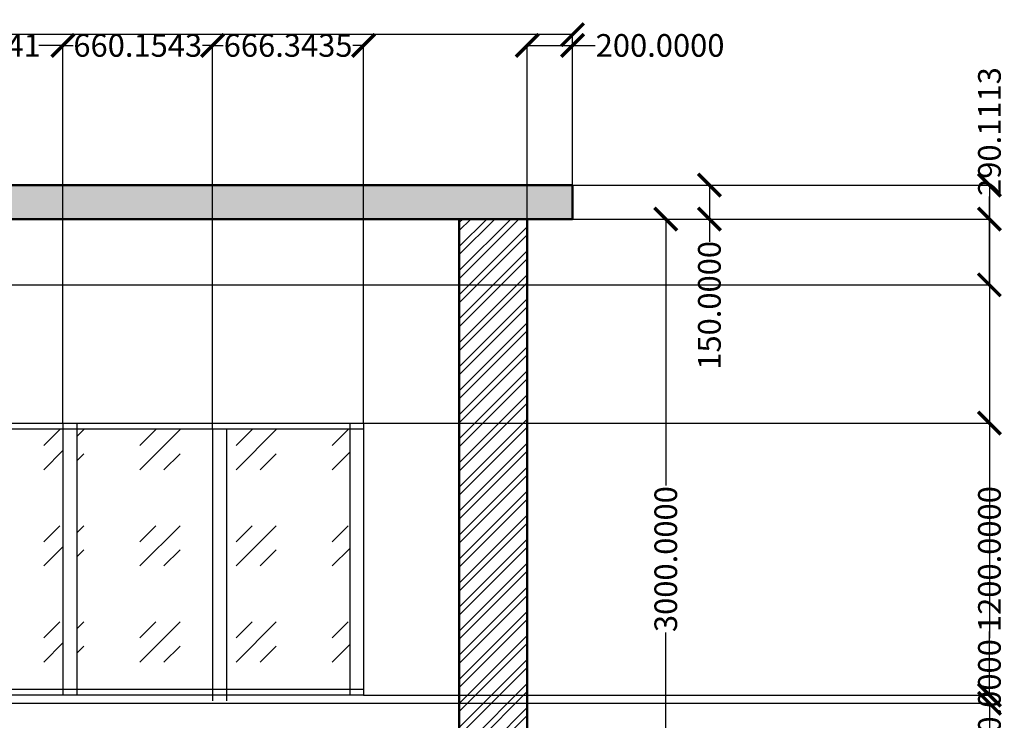
# Model space of a CAD drawing. Units: millimetres. Extents: x -4055 to 12299, y -682 to 5380.
# Tile 4 of 4: x 7955 to 12299, y 2289 to 5380. Entities that reach past the tile are written whole.
import ezdxf

# ---------------------------------------------------------------- set-up
doc = ezdxf.new("R2010")
doc.units = ezdxf.units.MM
doc.header["$MEASUREMENT"] = 0
for name, color, linetype, lineweight in [('A-ANNO-DIMS', 2, 'Continuous', 18), ('A-GLAZ', 4, 'Continuous', 25), ('A-GLAZ-PATT', 8, 'Continuous', 13), ('A-ROOF', 7, 'Continuous', 50), ('A-ROOF-PATT', 8, 'Continuous', 13), ('A-WALL', 7, 'Continuous', 50), ('A-WALL-PATT', 8, 'Continuous', 13)]:
    doc.layers.add(name, color=color, linetype=linetype, lineweight=lineweight)
doc.styles.get("Standard").update_dxf_attribs({"font": 'arial.ttf'})
doc.dimstyles.get("Standard").update_dxf_attribs({"dimtxt": 100, "dimasz": 100, "dimexe": 0.18, "dimexo": 0.0625, "dimgap": 0.09, "dimtad": 0, "dimdec": 4, "dimzin": 0, "dimdsep": 46, "dimtxsty": 'Standard', "dimblk": 'ARCHTICK', "dimcen": 0.09, "dimclrd": 3, "dimclre": 6, "dimclrt": 1, "dimadec": 0, "dimazin": 0, "dimtfac": 1, "dimtdec": 4, "dimtofl": 0, "dimtmove": 0, "dimatfit": 3, "dimfxl": 1, "dimtolj": 1, "dimtzin": 0, "dimlwd": 30, "dimarcsym": 0})

# ---------------------------------------------------------------- blocks, each defined once
blk = doc.blocks.new('_ArchTick')
at = {"color": 0, "linetype": 'ByBlock', "const_width": 0.15}
blk.add_lwpolyline([(-0.5, -0.5), (0.5, 0.5)], dxfattribs=at)
blk = doc.blocks.new('*D2')
at = {"layer": 'A-ANNO-DIMS', "color": 0, "lineweight": -2, "transparency": 16777216}
for p, q in [((10194.1, 4500), (10805.3, 4500)), ((10194.1, 1500), (10805.3, 1500))]:
    blk.add_line(p, q, dxfattribs=at)
at = {"layer": 'A-ANNO-DIMS', "color": 0, "lineweight": 30, "transparency": 16777216}
for p, q in [((10805.2, 4500), (10805.2, 3324)), ((10805.2, 1500), (10805.2, 2676))]:
    blk.add_line(p, q, dxfattribs=at)
at = {"layer": 'Defpoints', "color": 0, "transparency": 16777216}
for p in [(10194, 4500), (10194, 1500), (10805.2, 1500)]:
    blk.add_point(p, dxfattribs=at)
at = {"layer": 'A-ANNO-DIMS', "color": 0, "lineweight": 30, "transparency": 16777216, "xscale": 100, "yscale": 100, "zscale": 100}
for p, rotation in [((10805.2, 4500), 90), ((10805.2, 1500), 270)]:
    blk.add_blockref('_ArchTick', p, dxfattribs=dict(at, rotation=rotation))
at = {"layer": 'A-ANNO-DIMS', "color": 0, "transparency": 16777216, "insert": (10805.2, 3000), "char_height": 100, "attachment_point": 5, "rotation": 90}
blk.add_mtext('\\A1;3000.0000', dxfattribs=at)
blk = doc.blocks.new('*D11')
at = {"layer": 'A-ANNO-DIMS', "color": 0, "lineweight": -2, "transparency": 16777216}
for p, q in [((10394.1, 4650), (10997.8, 4650)), ((10394.1, 4500), (10997.8, 4500))]:
    blk.add_line(p, q, dxfattribs=at)
at = {"layer": 'A-ANNO-DIMS', "color": 0, "lineweight": 30, "transparency": 16777216}
for p, q in [((10997.7, 4650), (10997.7, 4500)), ((10997.7, 4500), (10997.7, 4400))]:
    blk.add_line(p, q, dxfattribs=at)
at = {"layer": 'Defpoints', "color": 0, "transparency": 16777216}
for p in [(10394, 4650), (10394, 4500), (10997.7, 4500)]:
    blk.add_point(p, dxfattribs=at)
at = {"layer": 'A-ANNO-DIMS', "color": 0, "lineweight": 30, "transparency": 16777216, "xscale": 100, "yscale": 100, "zscale": 100}
for p, rotation in [((10997.7, 4650), 90), ((10997.7, 4500), 270)]:
    blk.add_blockref('_ArchTick', p, dxfattribs=dict(at, rotation=rotation))
at = {"layer": 'A-ANNO-DIMS', "color": 0, "transparency": 16777216, "insert": (10997.7, 4119.5), "char_height": 100, "attachment_point": 5, "rotation": 90}
blk.add_mtext('\\A1;150.0000', dxfattribs=at)
blk = doc.blocks.new('*D12')
at = {"layer": 'A-ANNO-DIMS', "color": 0, "lineweight": -2, "transparency": 16777216}
for p, q in [((250, 4650.1), (250, 5314.3)), ((10394, 4650.1), (10394, 5314.3))]:
    blk.add_line(p, q, dxfattribs=at)
at = {"layer": 'A-ANNO-DIMS', "color": 0, "lineweight": 30, "transparency": 16777216}
for p, q in [((250, 5314.1), (4963.8, 5314.1)), ((10394, 5314.1), (5680.2, 5314.1))]:
    blk.add_line(p, q, dxfattribs=at)
at = {"layer": 'Defpoints', "color": 0, "transparency": 16777216}
for p in [(250, 5314.1), (250, 4650), (10394, 4650)]:
    blk.add_point(p, dxfattribs=at)
at = {"layer": 'A-ANNO-DIMS', "color": 0, "lineweight": 30, "transparency": 16777216, "xscale": 100, "yscale": 100, "zscale": 100, "rotation": 180}
blk.add_blockref('_ArchTick', (250, 5314.1), dxfattribs=at)
at = {"layer": 'A-ANNO-DIMS', "color": 0, "lineweight": 30, "transparency": 16777216, "xscale": 100, "yscale": 100, "zscale": 100}
blk.add_blockref('_ArchTick', (10394, 5314.1), dxfattribs=at)
at = {"layer": 'A-ANNO-DIMS', "color": 0, "transparency": 16777216, "insert": (5322, 5314.1), "char_height": 100, "attachment_point": 5}
blk.add_mtext('\\A1;10144.0310', dxfattribs=at)
blk = doc.blocks.new('*D19')
at = {"layer": 'A-ANNO-DIMS', "color": 6, "lineweight": -2, "transparency": 16777216}
for p, q in [((10394.1, 4650), (12233.2, 4650)), ((10644.1, 0), (12233.2, 0))]:
    blk.add_line(p, q, dxfattribs=at)
at = {"layer": 'A-ANNO-DIMS', "color": 3, "lineweight": 30, "transparency": 16777216}
for p, q in [((12233, 4650), (12233, 2651)), ((12233, 0), (12233, 1999))]:
    blk.add_line(p, q, dxfattribs=at)
at = {"layer": 'Defpoints', "color": 0, "transparency": 16777216}
for p in [(10394, 4650), (12233, 4650), (10644, 0)]:
    blk.add_point(p, dxfattribs=at)
at = {"layer": 'A-ANNO-DIMS', "color": 3, "lineweight": 30, "transparency": 16777216, "xscale": 100, "yscale": 100, "zscale": 100}
for p, rotation in [((12233, 4650), 90), ((12233, 0), 270)]:
    blk.add_blockref('_ArchTick', p, dxfattribs=dict(at, rotation=rotation))
at = {"layer": 'A-ANNO-DIMS', "color": 1, "transparency": 16777216, "insert": (12233, 2325), "char_height": 100, "attachment_point": 5, "rotation": 90}
blk.add_mtext('\\A1;4650.0000', dxfattribs=at)
blk = doc.blocks.new('*D22')
at = {"layer": 'A-ANNO-DIMS', "color": 6, "lineweight": -2, "transparency": 16777216}
for p, q in [((10194, 4500.1), (10194, 5266.4)), ((10394, 4650.1), (10394, 5266.4))]:
    blk.add_line(p, q, dxfattribs=at)
at = {"layer": 'A-ANNO-DIMS', "color": 3, "lineweight": 30, "transparency": 16777216}
for p, q in [((10194, 5266.2), (10394, 5266.2)), ((10394, 5266.2), (10494, 5266.2))]:
    blk.add_line(p, q, dxfattribs=at)
at = {"layer": 'Defpoints', "color": 0, "transparency": 16777216}
for p in [(10394, 5266.2), (10394, 4650), (10194, 4500)]:
    blk.add_point(p, dxfattribs=at)
at = {"layer": 'A-ANNO-DIMS', "color": 3, "lineweight": 30, "transparency": 16777216, "xscale": 100, "yscale": 100, "zscale": 100, "rotation": 180}
blk.add_blockref('_ArchTick', (10194, 5266.2), dxfattribs=at)
at = {"layer": 'A-ANNO-DIMS', "color": 3, "lineweight": 30, "transparency": 16777216, "xscale": 100, "yscale": 100, "zscale": 100}
blk.add_blockref('_ArchTick', (10394, 5266.2), dxfattribs=at)
at = {"layer": 'A-ANNO-DIMS', "color": 1, "transparency": 16777216, "insert": (10780.1, 5266.2), "char_height": 100, "attachment_point": 5}
blk.add_mtext('\\A1;200.0000', dxfattribs=at)
blk = doc.blocks.new('*D24')
at = {"layer": 'A-ANNO-DIMS', "color": 6, "lineweight": -2, "transparency": 16777216}
for p, q in [((7382.8, 3600.1), (7382.8, 5266.4)), ((8145.8, 3600.1), (8145.8, 5266.4))]:
    blk.add_line(p, q, dxfattribs=at)
at = {"layer": 'A-ANNO-DIMS', "color": 3, "lineweight": 30, "transparency": 16777216}
for p, q in [((7382.8, 5266.2), (7489, 5266.2)), ((8145.8, 5266.2), (8039.6, 5266.2))]:
    blk.add_line(p, q, dxfattribs=at)
at = {"layer": 'Defpoints', "color": 0, "transparency": 16777216}
for p in [(8145.8, 5266.2), (7382.8, 3600), (8145.8, 3600)]:
    blk.add_point(p, dxfattribs=at)
at = {"layer": 'A-ANNO-DIMS', "color": 3, "lineweight": 30, "transparency": 16777216, "xscale": 100, "yscale": 100, "zscale": 100, "rotation": 180}
blk.add_blockref('_ArchTick', (7382.8, 5266.2), dxfattribs=at)
at = {"layer": 'A-ANNO-DIMS', "color": 3, "lineweight": 30, "transparency": 16777216, "xscale": 100, "yscale": 100, "zscale": 100}
blk.add_blockref('_ArchTick', (8145.8, 5266.2), dxfattribs=at)
at = {"layer": 'A-ANNO-DIMS', "color": 1, "transparency": 16777216, "insert": (7764.3, 5266.2), "char_height": 100, "attachment_point": 5}
blk.add_mtext('\\A1;763.0741', dxfattribs=at)
blk = doc.blocks.new('*D25')
at = {"layer": 'A-ANNO-DIMS', "color": 6, "lineweight": -2, "transparency": 16777216}
for p, q in [((8145.8, 3600.1), (8145.8, 5266.4)), ((8806, 3575.1), (8806, 5266.4))]:
    blk.add_line(p, q, dxfattribs=at)
at = {"layer": 'A-ANNO-DIMS', "color": 3, "lineweight": 30, "transparency": 16777216}
for p, q in [((8145.8, 5266.2), (8190.3, 5266.2)), ((8806, 5266.2), (8761.5, 5266.2))]:
    blk.add_line(p, q, dxfattribs=at)
at = {"layer": 'Defpoints', "color": 0, "transparency": 16777216}
for p in [(8806, 5266.2), (8145.8, 3600), (8806, 3575)]:
    blk.add_point(p, dxfattribs=at)
at = {"layer": 'A-ANNO-DIMS', "color": 3, "lineweight": 30, "transparency": 16777216, "xscale": 100, "yscale": 100, "zscale": 100, "rotation": 180}
blk.add_blockref('_ArchTick', (8145.8, 5266.2), dxfattribs=at)
at = {"layer": 'A-ANNO-DIMS', "color": 3, "lineweight": 30, "transparency": 16777216, "xscale": 100, "yscale": 100, "zscale": 100}
blk.add_blockref('_ArchTick', (8806, 5266.2), dxfattribs=at)
at = {"layer": 'A-ANNO-DIMS', "color": 1, "transparency": 16777216, "insert": (8475.9, 5266.2), "char_height": 100, "attachment_point": 5}
blk.add_mtext('\\A1;660.1543', dxfattribs=at)
blk = doc.blocks.new('*D26')
at = {"layer": 'A-ANNO-DIMS', "color": 6, "lineweight": -2, "transparency": 16777216}
for p, q in [((8806, 3575.1), (8806, 5266.4)), ((9472.3, 3600.1), (9472.3, 5266.4))]:
    blk.add_line(p, q, dxfattribs=at)
at = {"layer": 'A-ANNO-DIMS', "color": 3, "lineweight": 30, "transparency": 16777216}
for p, q in [((8806, 5266.2), (8853.2, 5266.2)), ((9472.3, 5266.2), (9425.2, 5266.2))]:
    blk.add_line(p, q, dxfattribs=at)
at = {"layer": 'Defpoints', "color": 0, "transparency": 16777216}
for p in [(9472.3, 5266.2), (8806, 3575), (9472.3, 3600)]:
    blk.add_point(p, dxfattribs=at)
at = {"layer": 'A-ANNO-DIMS', "color": 3, "lineweight": 30, "transparency": 16777216, "xscale": 100, "yscale": 100, "zscale": 100, "rotation": 180}
blk.add_blockref('_ArchTick', (8806, 5266.2), dxfattribs=at)
at = {"layer": 'A-ANNO-DIMS', "color": 3, "lineweight": 30, "transparency": 16777216, "xscale": 100, "yscale": 100, "zscale": 100}
blk.add_blockref('_ArchTick', (9472.3, 5266.2), dxfattribs=at)
at = {"layer": 'A-ANNO-DIMS', "color": 1, "transparency": 16777216, "insert": (9139.2, 5266.2), "char_height": 100, "attachment_point": 5}
blk.add_mtext('\\A1;666.3435', dxfattribs=at)
blk = doc.blocks.new('*D27')
at = {"layer": 'A-ANNO-DIMS', "color": 6, "lineweight": -2, "transparency": 16777216}
for p, q in [((9472.4, 3600), (12233.2, 3600)), ((9472.4, 2400), (12233.2, 2400))]:
    blk.add_line(p, q, dxfattribs=at)
at = {"layer": 'A-ANNO-DIMS', "color": 3, "lineweight": 30, "transparency": 16777216}
for p, q in [((12233, 3600), (12233, 3319.3)), ((12233, 2400), (12233, 2680.7))]:
    blk.add_line(p, q, dxfattribs=at)
at = {"layer": 'Defpoints', "color": 0, "transparency": 16777216}
for p in [(9472.3, 3600), (12233, 3600), (9472.3, 2400)]:
    blk.add_point(p, dxfattribs=at)
at = {"layer": 'A-ANNO-DIMS', "color": 3, "lineweight": 30, "transparency": 16777216, "xscale": 100, "yscale": 100, "zscale": 100}
for p, rotation in [((12233, 3600), 90), ((12233, 2400), 270)]:
    blk.add_blockref('_ArchTick', p, dxfattribs=dict(at, rotation=rotation))
at = {"layer": 'A-ANNO-DIMS', "color": 1, "transparency": 16777216, "insert": (12233, 3000), "char_height": 100, "attachment_point": 5, "rotation": 90}
blk.add_mtext('\\A1;1200.0000', dxfattribs=at)
blk = doc.blocks.new('*D29')
at = {"layer": 'A-ANNO-DIMS', "color": 3, "lineweight": 30, "transparency": 16777216}
for p, q in [((12233, 4500), (12233, 4600)), ((12233, 4209.9), (12233, 4500))]:
    blk.add_line(p, q, dxfattribs=at)
at = {"layer": 'A-ANNO-DIMS', "color": 6, "lineweight": -2, "transparency": 16777216}
for p, q in [((750.1, 4500), (12233.2, 4500)), ((750.1, 4209.9), (12233.2, 4209.9))]:
    blk.add_line(p, q, dxfattribs=at)
at = {"layer": 'Defpoints', "color": 0, "transparency": 16777216}
for p in [(750, 4500), (12233, 4500), (750, 4209.9)]:
    blk.add_point(p, dxfattribs=at)
at = {"layer": 'A-ANNO-DIMS', "color": 3, "lineweight": 30, "transparency": 16777216, "xscale": 100, "yscale": 100, "zscale": 100}
for p, rotation in [((12233, 4500), 90), ((12233, 4209.9), 270)]:
    blk.add_blockref('_ArchTick', p, dxfattribs=dict(at, rotation=rotation))
at = {"layer": 'A-ANNO-DIMS', "color": 1, "transparency": 16777216, "insert": (12233, 4886.2), "char_height": 100, "attachment_point": 5, "rotation": 90}
blk.add_mtext('\\A1;290.1113', dxfattribs=at)
blk = doc.blocks.new('*D34')
at = {"layer": 'A-ANNO-DIMS', "color": 6, "lineweight": -2, "transparency": 16777216}
for p, q in [((6374.7, 2363.8), (12233.2, 2363.8)), ((6374.7, 1500), (12233.2, 1500))]:
    blk.add_line(p, q, dxfattribs=at)
at = {"layer": 'A-ANNO-DIMS', "color": 3, "lineweight": 30, "transparency": 16777216}
for p, q in [((12233, 2363.8), (12233, 2217.3)), ((12233, 1500), (12233, 1646.5))]:
    blk.add_line(p, q, dxfattribs=at)
at = {"layer": 'Defpoints', "color": 0, "transparency": 16777216}
for p in [(6374.6, 2363.8), (12233, 2363.8), (6374.6, 1500)]:
    blk.add_point(p, dxfattribs=at)
at = {"layer": 'A-ANNO-DIMS', "color": 3, "lineweight": 30, "transparency": 16777216, "xscale": 100, "yscale": 100, "zscale": 100}
for p, rotation in [((12233, 2363.8), 90), ((12233, 1500), 270)]:
    blk.add_blockref('_ArchTick', p, dxfattribs=dict(at, rotation=rotation))
at = {"layer": 'A-ANNO-DIMS', "color": 1, "transparency": 16777216, "insert": (12233, 1931.9), "char_height": 100, "attachment_point": 5, "rotation": 90}
blk.add_mtext('\\A1;863.7746', dxfattribs=at)

msp = doc.modelspace()

# ---------------------------------------------------------------- hatches: boundary and pattern name
at = {"layer": 'A-GLAZ-PATT'}
h = msp.add_hatch(dxfattribs=at)
h.set_pattern_fill('GOST_GLASS', color=256, scale=50)
h.set_pattern_definition([(45, (0, 0), (424.264, 0), [250, -350]), (45, (106.07, 0), (424.264, 0), [100, -500]), (45, (0, 106.07), (424.264, 0), [100, -500])])
h.paths.add_polyline_path([(7382.76217, 3575), (6394.60797, 3575), (6394.60797, 2423.65166), (7382.76163, 2424.08457)])
h.paths.add_polyline_path([(8145.83628, 3575), (7444.13336, 3575), (7444.13282, 2424.11146), (8145.83574, 2424.41887)])
h.paths.add_polyline_path([(8805.9906, 3575), (8207.20748, 3575), (8207.20694, 2424.44576), (8805.99007, 2424.70808)])
h.paths.add_polyline_path([(9410.96289, 3575), (8867.3618, 3575), (8867.36126, 2424.73497), (9410.96235, 2424.97312)])
at = {"layer": 'A-ROOF-PATT'}
h = msp.add_hatch(dxfattribs=at)
h.set_pattern_fill('AR-CONC', color=256, scale=20)
h.set_pattern_definition([(50, (0, 0), (143.452, -12.5504), [15, -165]), (355, (0, 0), (-27.7503, 150.4384), [12, -132]), (100.4514, (11.95, -1.05), (115.7018, 137.888), [12.748, -140.2284]), (46.1842, (0, 40), (213.4483, -33.1039), [22.5, -247.5]), (96.6356, (17.79, 37.24), (186.9324, 194.8237), [19.122, -210.3428]), (351.1842, (0, 40), (186.9324, 194.8237), [18, -198]), (21, (20, 30), (119.3814, -80.5238), [15, -165]), (326, (20, 30), (48.663, 145.03), [12, -132]), (71.4514, (29.95, 23.29), (168.0445, 64.5062), [12.748, -140.2284]), (37.5, (0, 0), (2.43197, 66.57877), [0, -130.4, 0, -134, 0, -132.5]), (7.5, (0, 0), (52.6139, 78.88234), [0, -76.4, 0, -127.4, 0, -50.5]), (327.5, (-44.6, 0), (106.76449, -4.51097), [0, -50, 0, -156, 0, -207]), (317.5, (-64.6, 0), (116.6372, 20.021), [0, -65, 0, -103.6, 0, -147])])
h.paths.add_polyline_path([(10394.03102, 4650), (250, 4650), (250, 4500), (10394.03102, 4500)])
at = {"layer": 'A-WALL-PATT'}
h = msp.add_hatch(dxfattribs=at)
h.set_pattern_fill('ANSI32', color=256, scale=200)
h.paths.add_polyline_path([(750, 3719.22559), (450, 3719.22559), (450, 1500), (750, 1500)])
h.paths.add_polyline_path([(3378.64487, 4500), (3078.64487, 4500), (3078.64487, 1500), (3378.64487, 1500)])
h.paths.add_polyline_path([(5194.60797, 4500), (4894.60797, 4500), (4894.60797, 1500), (5194.60797, 1500), (5194.60797, 3600)])
h.paths.add_polyline_path([(750, 4500), (450, 4500), (450, 4209.88871), (750, 4209.88871)])
h.paths.add_polyline_path([(10194.03102, 4500), (9894.03102, 4500), (9894.03102, 1500), (10194.03102, 1500)])

# ---------------------------------------------------------------- linework, layer by layer
at = {"layer": 'A-GLAZ'}
for p, q in [((6394.60797, 3600), (9472.33409, 3600)), ((6394.60797, 3575), (9472.33409, 3575)), ((8145.83629, 3600), (8145.83573, 2399.08457)), ((8207.20749, 3600), (8207.20692, 2399.08457)), ((8805.9906, 3575), (8805.99004, 2374.08457)), ((8867.3618, 3575), (8867.36123, 2374.08457)), ((9410.9629, 3600), (9410.96234, 2399.08457)), ((9472.33409, 3600), (9472.33353, 2399.08457)), ((9472.33409, 3600), (9472.33409, 2400)), ((9472.32314, 2425), (6394.59702, 2423.65166)), ((9472.33409, 2400), (6394.60797, 2398.65166))]:
    msp.add_line(p, q, dxfattribs=at)
at = {"layer": 'A-ROOF'}
for p, q in [((10394.03102, 4650), (250, 4650)), ((10394.03102, 4500), (10394.03102, 4650)), ((250, 4500), (10394.03102, 4500))]:
    msp.add_line(p, q, dxfattribs=at)
at = {"layer": 'A-WALL'}
for p, q in [((9894.03102, 1500), (9894.03102, 4500)), ((9894.03102, 4500), (10194.03102, 4500)), ((10194.03102, 4500), (10194.03102, 1500))]:
    msp.add_line(p, q, dxfattribs=at)

# ---------------------------------------------------------------- dimensions: what is measured, and where the dimension line sits
at = {"layer": 'A-ANNO-DIMS'}
for base, p1, p2, override, picture, middle in [((250, 5314.10321), (10394.03102, 4650), (250, 4650), {"dimclrd": 0, "dimclre": 0, "dimclrt": 0}, '*D12', (5322.01551, 5314.10321)), ((8145.83629, 5266.25), (7382.76218, 3600), (8145.83629, 3600), {"dimdec": 4, "dimlfac": 1, "dimrnd": 0, "dimzin": 0, "dimdsep": 46, "dimlunit": 2}, '*D24', (7764.29924, 5266.25)), ((8805.99061, 5266.25), (8145.83629, 3600), (8805.99061, 3575), {"dimdec": 4, "dimlfac": 1, "dimrnd": 0, "dimzin": 0, "dimdsep": 46, "dimlunit": 2}, '*D25', (8475.91345, 5266.25)), ((9472.33409, 5266.25), (8805.99061, 3575), (9472.33409, 3600), {"dimdec": 4, "dimlfac": 1, "dimrnd": 0, "dimzin": 0, "dimdsep": 46, "dimlunit": 2}, '*D26', (9139.16235, 5266.25)), ((10394.03102, 5266.25), (10194.03102, 4500), (10394.03102, 4650), {"dimdec": 4, "dimlfac": 1, "dimrnd": 0, "dimzin": 0, "dimdsep": 46, "dimlunit": 2}, '*D22', (10780.06918, 5266.25))]:
    dim = msp.add_linear_dim(base=base, p1=p1, p2=p2, dimstyle='Standard', override=override, dxfattribs=at)
    dim.commit()
    dim.dimension.update_dxf_attribs({"geometry": picture, "text_midpoint": middle})
for base, p1, p2, override, picture, middle in [((12232.99644, 4500), (750, 4209.88871), (750, 4500), {"dimdec": 4, "dimlfac": 1, "dimrnd": 0, "dimzin": 0, "dimdsep": 46, "dimlunit": 2}, '*D29', (12232.99644, 4886.20869)), ((10997.66779, 4500), (10394.03102, 4650), (10394.03102, 4500), {"dimclrd": 0, "dimclre": 0, "dimclrt": 0}, '*D11', (10997.66779, 4119.52119)), ((12232.99644, 4650), (10644.03102, 0), (10394.03102, 4650), {"dimdec": 4, "dimlfac": 1, "dimrnd": 0, "dimzin": 0, "dimdsep": 46, "dimlunit": 2}, '*D19', (12232.99644, 2325)), ((10805.16529, 1500), (10194.03102, 4500), (10194.03102, 1500), {"dimclrd": 0, "dimclre": 0, "dimclrt": 0}, '*D2', (10805.16529, 3000)), ((12232.99644, 3600), (9472.33409, 2400), (9472.33409, 3600), {"dimdec": 4, "dimlfac": 1, "dimrnd": 0, "dimzin": 0, "dimdsep": 46, "dimlunit": 2}, '*D27', (12232.99644, 3000)), ((12232.99644, 2363.77463), (6374.60797, 1500), (6374.60797, 2363.77463), {"dimdec": 4, "dimlfac": 1, "dimrnd": 0, "dimzin": 0, "dimdsep": 46, "dimlunit": 2}, '*D34', (12232.99644, 1931.88731))]:
    dim = msp.add_linear_dim(base=base, p1=p1, p2=p2, angle=90, dimstyle='Standard', override=override, dxfattribs=at)
    dim.commit()
    dim.dimension.update_dxf_attribs({"geometry": picture, "text_midpoint": middle})

doc.saveas('drawing.dxf')
